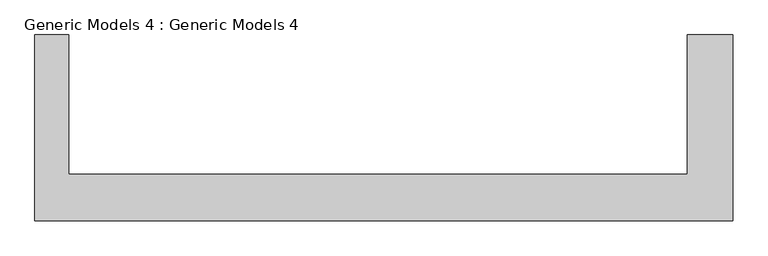
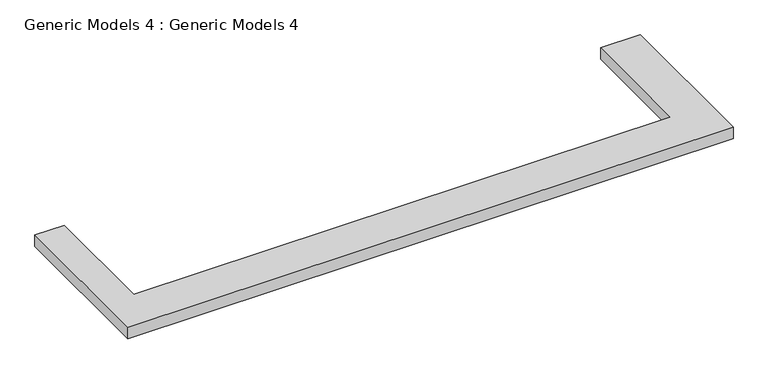
"""IFC4 building model written with IfcOpenShell, lengths in millimetres: proxy geometry, Generic Models 4 : Generic Models 4."""

from ifc_helpers import new_model, si_unit, frame, origin, place, context, project, spatial, polyline, outline, extrude, source, transform, mapped, element, save


def generic_models_4_generic_models_4_79451922(model_context):
    return source(origin(), model_context, "Body", "SweptSolid", [
        extrude(outline(polyline([(-16282.4255016, -15522.0678064), (-16282.4255016, -14848.9678064), (-16160.2775602, -14848.9678064), (-16160.2775602, -15353.4653967), (-13918.3150098, -15353.4653967), (-13918.3150098, -14848.9678064), (-13753.2020297, -14848.9678064), (-13753.2020297, -15522.0678064), (-16282.4255016, -15522.0678064)])), frame((0.0, 0.0, 7629.8225171), z_axis=(0.0, 0.0, 1.0), x_axis=(1.0, 0.0, 0.0)), (0.0, 0.0, 1.0), 50.8),
    ])


if __name__ == "__main__":
    model = new_model("IFC4")
    model_context = context("Model", 3, world=origin())
    ifc_project = project(units=[si_unit("LENGTHUNIT", "METRE", prefix="MILLI")], contexts=[model_context])
    site = spatial("IfcSite", under=ifc_project)
    building = spatial("IfcBuilding", under=site)
    placement = place(None, origin())
    generic_models_4_generic_models_4_shape = generic_models_4_generic_models_4_79451922(model_context)
    element("IfcBuildingElementProxy", 1, Name="Generic Models 4 : Generic Models 4", ObjectType="Generic Models 4 : Generic Models 4", at=placement, inside=building, context=model_context, shape_type="MappedRepresentation", body=[
        mapped(generic_models_4_generic_models_4_shape, transform((0.0, 0.0, 0.0), x_axis=(1.0, 0.0, 0.0), y_axis=(0.0, 1.0, 0.0), z_axis=(0.0, 0.0, 1.0))),
    ])
    save(model, "model.ifc")
